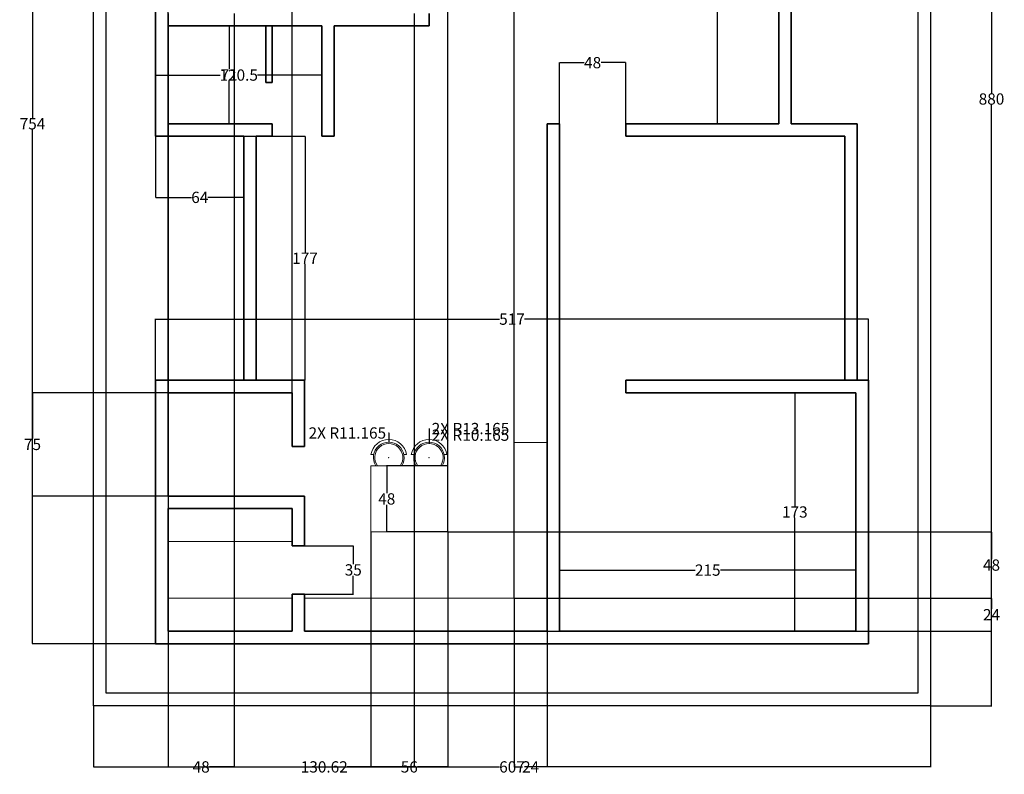
# Model space of a CAD drawing. Units: inches. Extents: x -254 to 1961, y 86 to 3025.
# Tile 5 of 6: x 1247 to 1961, y 2046 to 2593. Entities that reach past the tile are written whole.
import ezdxf

# ---------------------------------------------------------------- set-up
doc = ezdxf.new("R2010")
doc.units = ezdxf.units.IN
doc.header["$MEASUREMENT"] = 0
for name, color, linetype, lineweight in [('A-ANNO-DIMS', 2, 'Continuous', 18), ('C-SITE-WALL', 8, 'Continuous', 30), ('FURNITURE', 151, 'Continuous', 13), ('KITCHEN', 9, 'Continuous', 18), ('WALLS', 255, 'Continuous', 35)]:
    doc.layers.add(name, color=color, linetype=linetype, lineweight=lineweight)
doc.styles.get("Standard").update_dxf_attribs({"font": 'arial.ttf'})
doc.dimstyles.get("Standard").update_dxf_attribs({"dimtxt": 8.18, "dimasz": 0.18, "dimexe": 0.18, "dimexo": 0.0625, "dimgap": 0.09, "dimtad": 0, "dimtih": 1, "dimtoh": 1, "dimdec": 1, "dimzin": 0, "dimdsep": 46, "dimlunit": 3, "dimtxsty": 'Standard', "dimcen": 0.09, "dimadec": 0, "dimazin": 0, "dimtfac": 1, "dimtdec": 1, "dimtofl": 0, "dimtmove": 0, "dimatfit": 3, "dimfxl": 1, "dimtolj": 1, "dimtzin": 0, "dimarcsym": 0})

# ---------------------------------------------------------------- blocks, each defined once
blk = doc.blocks.new('*D71')
at = {"layer": 'A-ANNO-DIMS', "color": 0, "lineweight": -2, "transparency": 16777216}
for p, q in [((1300.37, 2095.39), (1300.37, 2050.93)), ((1907.37, 2095.39), (1907.37, 2050.93)), ((1300.55, 2051.11), (1594.72, 2051.11)), ((1907.19, 2051.11), (1613.02, 2051.11))]:
    blk.add_line(p, q, dxfattribs=at)
at = {"layer": 'A-ANNO-DIMS', "color": 0, "transparency": 16777216}
for points in [[(1300.55, 2051.14), (1300.55, 2051.08), (1300.37, 2051.11)], [(1907.19, 2051.14), (1907.19, 2051.08), (1907.37, 2051.11)]]:
    blk.add_solid(points, dxfattribs=at)
at = {"layer": 'Defpoints', "color": 0, "transparency": 16777216}
for p in [(1300.37, 2095.46), (1907.37, 2095.46), (1907.37, 2051.11)]:
    blk.add_point(p, dxfattribs=at)
at = {"layer": 'A-ANNO-DIMS', "color": 0, "transparency": 16777216, "insert": (1603.87, 2051.11), "char_height": 8.18, "attachment_point": 5}
blk.add_mtext('\\A1;607', dxfattribs=at)
blk = doc.blocks.new('*D72')
at = {"layer": 'A-ANNO-DIMS', "color": 0, "lineweight": -2, "transparency": 16777216}
for p, q in [((1907.43, 2975.46), (1951.9, 2975.46)), ((1951.72, 2975.28), (1951.72, 2539.72)), ((1951.72, 2095.64), (1951.72, 2531.19)), ((1907.43, 2095.46), (1951.9, 2095.46))]:
    blk.add_line(p, q, dxfattribs=at)
at = {"layer": 'A-ANNO-DIMS', "color": 0, "transparency": 16777216}
for points in [[(1951.69, 2975.28), (1951.75, 2975.28), (1951.72, 2975.46)], [(1951.69, 2095.64), (1951.75, 2095.64), (1951.72, 2095.46)]]:
    blk.add_solid(points, dxfattribs=at)
at = {"layer": 'Defpoints', "color": 0, "transparency": 16777216}
for p in [(1907.37, 2975.46), (1951.72, 2975.46), (1907.37, 2095.46)]:
    blk.add_point(p, dxfattribs=at)
at = {"layer": 'A-ANNO-DIMS', "color": 0, "transparency": 16777216, "insert": (1951.72, 2535.46), "char_height": 8.18, "attachment_point": 5}
blk.add_mtext('\\A1;880', dxfattribs=at)
blk = doc.blocks.new('*D73')
at = {"layer": 'A-ANNO-DIMS', "color": 0, "lineweight": -2, "transparency": 16777216}
for p, q in [((1345.37, 2331.52), (1345.37, 2375.99)), ((1345.55, 2375.81), (1594.74, 2375.81)), ((1862.19, 2375.81), (1613, 2375.81)), ((1862.37, 2331.52), (1862.37, 2375.99))]:
    blk.add_line(p, q, dxfattribs=at)
at = {"layer": 'A-ANNO-DIMS', "color": 0, "transparency": 16777216}
for points in [[(1345.55, 2375.84), (1345.55, 2375.78), (1345.37, 2375.81)], [(1862.19, 2375.84), (1862.19, 2375.78), (1862.37, 2375.81)]]:
    blk.add_solid(points, dxfattribs=at)
at = {"layer": 'Defpoints', "color": 0, "transparency": 16777216}
for p in [(1862.37, 2375.81), (1345.37, 2331.46), (1862.37, 2331.46)]:
    blk.add_point(p, dxfattribs=at)
at = {"layer": 'A-ANNO-DIMS', "color": 0, "transparency": 16777216, "insert": (1603.87, 2375.81), "char_height": 8.18, "attachment_point": 5}
blk.add_mtext('\\A1;517', dxfattribs=at)
blk = doc.blocks.new('*D74')
at = {"layer": 'A-ANNO-DIMS', "color": 0, "lineweight": -2, "transparency": 16777216}
for p, q in [((1345.31, 2894.46), (1255.84, 2894.46)), ((1256.02, 2894.28), (1256.02, 2521.71)), ((1256.02, 2140.64), (1256.02, 2513.21)), ((1345.31, 2140.46), (1255.84, 2140.46))]:
    blk.add_line(p, q, dxfattribs=at)
at = {"layer": 'A-ANNO-DIMS', "color": 0, "transparency": 16777216}
for points in [[(1255.99, 2894.28), (1256.05, 2894.28), (1256.02, 2894.46)], [(1255.99, 2140.64), (1256.05, 2140.64), (1256.02, 2140.46)]]:
    blk.add_solid(points, dxfattribs=at)
at = {"layer": 'Defpoints', "color": 0, "transparency": 16777216}
for p in [(1256.02, 2894.46), (1345.37, 2894.46), (1345.37, 2140.46)]:
    blk.add_point(p, dxfattribs=at)
at = {"layer": 'A-ANNO-DIMS', "color": 0, "transparency": 16777216, "insert": (1256.02, 2517.46), "char_height": 8.18, "attachment_point": 5}
blk.add_mtext('\\A1;754', dxfattribs=at)
blk = doc.blocks.new('*D87')
at = {"layer": 'A-ANNO-DIMS', "color": 0, "lineweight": -2, "transparency": 16777216}
for p, q in [((1797.31, 2753.46), (1752.84, 2753.46)), ((1753.02, 2753.28), (1753.02, 2639.72)), ((1753.02, 2517.64), (1753.02, 2631.19)), ((1797.31, 2517.46), (1752.84, 2517.46))]:
    blk.add_line(p, q, dxfattribs=at)
at = {"layer": 'A-ANNO-DIMS', "color": 0, "transparency": 16777216}
for points in [[(1752.99, 2753.28), (1753.05, 2753.28), (1753.02, 2753.46)], [(1752.99, 2517.64), (1753.05, 2517.64), (1753.02, 2517.46)]]:
    blk.add_solid(points, dxfattribs=at)
at = {"layer": 'Defpoints', "color": 0, "transparency": 16777216}
for p in [(1753.02, 2753.46), (1797.37, 2753.46), (1797.37, 2517.46)]:
    blk.add_point(p, dxfattribs=at)
at = {"layer": 'A-ANNO-DIMS', "color": 0, "transparency": 16777216, "insert": (1753.02, 2635.46), "char_height": 8.18, "attachment_point": 5}
blk.add_mtext('\\A1;236', dxfattribs=at)
blk = doc.blocks.new('*D88')
at = {"layer": 'A-ANNO-DIMS', "color": 0, "lineweight": -2, "transparency": 16777216}
for p, q in [((1409.43, 2508.46), (1453.9, 2508.46)), ((1453.72, 2508.28), (1453.72, 2424.15)), ((1453.72, 2331.64), (1453.72, 2415.76)), ((1409.43, 2331.46), (1453.9, 2331.46))]:
    blk.add_line(p, q, dxfattribs=at)
at = {"layer": 'A-ANNO-DIMS', "color": 0, "transparency": 16777216}
for points in [[(1453.69, 2508.28), (1453.75, 2508.28), (1453.72, 2508.46)], [(1453.69, 2331.64), (1453.75, 2331.64), (1453.72, 2331.46)]]:
    blk.add_solid(points, dxfattribs=at)
at = {"layer": 'Defpoints', "color": 0, "transparency": 16777216}
for p in [(1409.37, 2508.46), (1409.37, 2331.46), (1453.72, 2331.46)]:
    blk.add_point(p, dxfattribs=at)
at = {"layer": 'A-ANNO-DIMS', "color": 0, "transparency": 16777216, "insert": (1453.72, 2419.96), "char_height": 8.18, "attachment_point": 5}
blk.add_mtext('\\A1;177', dxfattribs=at)
blk = doc.blocks.new('*D89')
at = {"layer": 'A-ANNO-DIMS', "color": 0, "lineweight": -2, "transparency": 16777216}
for p, q in [((1345.37, 2508.39), (1345.37, 2463.93)), ((1409.37, 2508.39), (1409.37, 2463.93)), ((1345.55, 2464.11), (1371.41, 2464.11)), ((1409.19, 2464.11), (1383.32, 2464.11))]:
    blk.add_line(p, q, dxfattribs=at)
at = {"layer": 'A-ANNO-DIMS', "color": 0, "transparency": 16777216}
for points in [[(1345.55, 2464.14), (1345.55, 2464.08), (1345.37, 2464.11)], [(1409.19, 2464.14), (1409.19, 2464.08), (1409.37, 2464.11)]]:
    blk.add_solid(points, dxfattribs=at)
at = {"layer": 'Defpoints', "color": 0, "transparency": 16777216}
for p in [(1345.37, 2508.46), (1409.37, 2508.46), (1345.37, 2464.11)]:
    blk.add_point(p, dxfattribs=at)
at = {"layer": 'A-ANNO-DIMS', "color": 0, "transparency": 16777216, "insert": (1377.37, 2464.11), "char_height": 8.18, "attachment_point": 5}
blk.add_mtext('\\A1;64', dxfattribs=at)
blk = doc.blocks.new('*D90')
at = {"layer": 'A-ANNO-DIMS', "color": 0, "lineweight": -2, "transparency": 16777216}
for p, q in [((1638.37, 2149.52), (1638.37, 2193.99)), ((1638.55, 2193.81), (1736.64, 2193.81)), ((1853.19, 2193.81), (1755.1, 2193.81)), ((1853.37, 2149.52), (1853.37, 2193.99))]:
    blk.add_line(p, q, dxfattribs=at)
at = {"layer": 'A-ANNO-DIMS', "color": 0, "transparency": 16777216}
for points in [[(1638.55, 2193.84), (1638.55, 2193.78), (1638.37, 2193.81)], [(1853.19, 2193.84), (1853.19, 2193.78), (1853.37, 2193.81)]]:
    blk.add_solid(points, dxfattribs=at)
at = {"layer": 'Defpoints', "color": 0, "transparency": 16777216}
for p in [(1853.37, 2193.81), (1638.37, 2149.46), (1853.37, 2149.46)]:
    blk.add_point(p, dxfattribs=at)
at = {"layer": 'A-ANNO-DIMS', "color": 0, "transparency": 16777216, "insert": (1745.87, 2193.81), "char_height": 8.18, "attachment_point": 5}
blk.add_mtext('\\A1;215', dxfattribs=at)
blk = doc.blocks.new('*D91')
at = {"layer": 'A-ANNO-DIMS', "color": 0, "lineweight": -2, "transparency": 16777216}
for p, q in [((1853.31, 2322.46), (1808.84, 2322.46)), ((1809.02, 2322.28), (1809.02, 2240.22)), ((1809.02, 2149.64), (1809.02, 2231.69)), ((1853.31, 2149.46), (1808.84, 2149.46))]:
    blk.add_line(p, q, dxfattribs=at)
at = {"layer": 'A-ANNO-DIMS', "color": 0, "transparency": 16777216}
for points in [[(1808.99, 2322.28), (1809.05, 2322.28), (1809.02, 2322.46)], [(1808.99, 2149.64), (1809.05, 2149.64), (1809.02, 2149.46)]]:
    blk.add_solid(points, dxfattribs=at)
at = {"layer": 'Defpoints', "color": 0, "transparency": 16777216}
for p in [(1809.02, 2322.46), (1853.37, 2322.46), (1853.37, 2149.46)]:
    blk.add_point(p, dxfattribs=at)
at = {"layer": 'A-ANNO-DIMS', "color": 0, "transparency": 16777216, "insert": (1809.02, 2235.96), "char_height": 8.18, "attachment_point": 5}
blk.add_mtext('\\A1;173', dxfattribs=at)
blk = doc.blocks.new('*D92')
at = {"layer": 'A-ANNO-DIMS', "color": 0, "lineweight": -2, "transparency": 16777216}
for p, q in [((1638.37, 2517.52), (1638.37, 2561.99)), ((1638.55, 2561.81), (1656.25, 2561.81)), ((1686.19, 2561.81), (1668.49, 2561.81)), ((1686.37, 2517.52), (1686.37, 2561.99))]:
    blk.add_line(p, q, dxfattribs=at)
at = {"layer": 'A-ANNO-DIMS', "color": 0, "transparency": 16777216}
for points in [[(1638.55, 2561.84), (1638.55, 2561.78), (1638.37, 2561.81)], [(1686.19, 2561.84), (1686.19, 2561.78), (1686.37, 2561.81)]]:
    blk.add_solid(points, dxfattribs=at)
at = {"layer": 'Defpoints', "color": 0, "transparency": 16777216}
for p in [(1686.37, 2561.81), (1638.37, 2517.46), (1686.37, 2517.46)]:
    blk.add_point(p, dxfattribs=at)
at = {"layer": 'A-ANNO-DIMS', "color": 0, "transparency": 16777216, "insert": (1662.37, 2561.81), "char_height": 8.18, "attachment_point": 5}
blk.add_mtext('\\A1;48', dxfattribs=at)
blk = doc.blocks.new('*D93')
at = {"layer": 'A-ANNO-DIMS', "color": 0, "lineweight": -2, "transparency": 16777216}
for p, q in [((1402.37, 2597.39), (1402.37, 2050.93)), ((1532.98, 2597.39), (1532.98, 2050.93)), ((1402.55, 2051.11), (1451.03, 2051.11)), ((1532.8, 2051.11), (1484.32, 2051.11))]:
    blk.add_line(p, q, dxfattribs=at)
at = {"layer": 'A-ANNO-DIMS', "color": 0, "transparency": 16777216}
for points in [[(1402.55, 2051.14), (1402.55, 2051.08), (1402.37, 2051.11)], [(1532.8, 2051.14), (1532.8, 2051.08), (1532.98, 2051.11)]]:
    blk.add_solid(points, dxfattribs=at)
at = {"layer": 'Defpoints', "color": 0, "transparency": 16777216}
for p in [(1402.37, 2597.46), (1532.98, 2597.46), (1532.98, 2051.11)]:
    blk.add_point(p, dxfattribs=at)
at = {"layer": 'A-ANNO-DIMS', "color": 0, "transparency": 16777216, "insert": (1467.68, 2051.11), "char_height": 8.18, "attachment_point": 5}
blk.add_mtext('\\A1;130.62', dxfattribs=at)
blk = doc.blocks.new('*D94')
at = {"layer": 'A-ANNO-DIMS', "color": 0, "lineweight": -2, "transparency": 16777216}
for p, q in [((1354.37, 2597.39), (1354.37, 2050.93)), ((1402.37, 2597.39), (1402.37, 2050.93)), ((1354.55, 2051.11), (1372.25, 2051.11)), ((1402.19, 2051.11), (1384.49, 2051.11))]:
    blk.add_line(p, q, dxfattribs=at)
at = {"layer": 'A-ANNO-DIMS', "color": 0, "transparency": 16777216}
for points in [[(1354.55, 2051.14), (1354.55, 2051.08), (1354.37, 2051.11)], [(1402.19, 2051.14), (1402.19, 2051.08), (1402.37, 2051.11)]]:
    blk.add_solid(points, dxfattribs=at)
at = {"layer": 'Defpoints', "color": 0, "transparency": 16777216}
for p in [(1354.37, 2597.46), (1402.37, 2597.46), (1402.37, 2051.11)]:
    blk.add_point(p, dxfattribs=at)
at = {"layer": 'A-ANNO-DIMS', "color": 0, "transparency": 16777216, "insert": (1378.37, 2051.11), "char_height": 8.18, "attachment_point": 5}
blk.add_mtext('\\A1;48', dxfattribs=at)
blk = doc.blocks.new('*D99')
at = {"layer": 'A-ANNO-DIMS', "color": 0, "lineweight": -2, "transparency": 16777216}
for p, q in [((1345.37, 2508.52), (1345.37, 2552.99)), ((1345.55, 2552.81), (1392.08, 2552.81)), ((1465.69, 2552.81), (1419.16, 2552.81)), ((1465.87, 2508.52), (1465.87, 2552.99))]:
    blk.add_line(p, q, dxfattribs=at)
at = {"layer": 'A-ANNO-DIMS', "color": 0, "transparency": 16777216}
for points in [[(1345.55, 2552.84), (1345.55, 2552.78), (1345.37, 2552.81)], [(1465.69, 2552.84), (1465.69, 2552.78), (1465.87, 2552.81)]]:
    blk.add_solid(points, dxfattribs=at)
at = {"layer": 'Defpoints', "color": 0, "transparency": 16777216}
for p in [(1465.87, 2552.81), (1345.37, 2508.46), (1465.87, 2508.46)]:
    blk.add_point(p, dxfattribs=at)
at = {"layer": 'A-ANNO-DIMS', "color": 0, "transparency": 16777216, "insert": (1405.62, 2552.81), "char_height": 8.18, "attachment_point": 5}
blk.add_mtext('\\A1;120.5', dxfattribs=at)
blk = doc.blocks.new('*D100')
at = {"layer": 'A-ANNO-DIMS', "color": 0, "lineweight": -2, "transparency": 16777216}
for p, q in [((1354.43, 2588.46), (1398.9, 2588.46)), ((1398.72, 2588.28), (1398.72, 2557.15)), ((1398.72, 2517.64), (1398.72, 2548.76)), ((1354.43, 2517.46), (1398.9, 2517.46))]:
    blk.add_line(p, q, dxfattribs=at)
at = {"layer": 'A-ANNO-DIMS', "color": 0, "transparency": 16777216}
for points in [[(1398.69, 2588.28), (1398.75, 2588.28), (1398.72, 2588.46)], [(1398.69, 2517.64), (1398.75, 2517.64), (1398.72, 2517.46)]]:
    blk.add_solid(points, dxfattribs=at)
at = {"layer": 'Defpoints', "color": 0, "transparency": 16777216}
for p in [(1354.37, 2588.46), (1354.37, 2517.46), (1398.72, 2517.46)]:
    blk.add_point(p, dxfattribs=at)
at = {"layer": 'A-ANNO-DIMS', "color": 0, "transparency": 16777216, "insert": (1398.72, 2552.96), "char_height": 8.18, "attachment_point": 5}
blk.add_mtext('\\A1;71', dxfattribs=at)
blk = doc.blocks.new('*D104')
at = {"layer": 'A-ANNO-DIMS', "color": 0, "lineweight": -2, "transparency": 16777216}
for p, q in [((1354.37, 2322.52), (1354.37, 3019.99)), ((1354.55, 3019.81), (1393.43, 3019.81)), ((1444.19, 3019.81), (1405.3, 3019.81)), ((1444.37, 2322.52), (1444.37, 3019.99))]:
    blk.add_line(p, q, dxfattribs=at)
at = {"layer": 'A-ANNO-DIMS', "color": 0, "transparency": 16777216}
for points in [[(1354.55, 3019.84), (1354.55, 3019.78), (1354.37, 3019.81)], [(1444.19, 3019.84), (1444.19, 3019.78), (1444.37, 3019.81)]]:
    blk.add_solid(points, dxfattribs=at)
at = {"layer": 'Defpoints', "color": 0, "transparency": 16777216}
for p in [(1444.37, 3019.81), (1354.37, 2322.46), (1444.37, 2322.46)]:
    blk.add_point(p, dxfattribs=at)
at = {"layer": 'A-ANNO-DIMS', "color": 0, "transparency": 16777216, "insert": (1399.37, 3019.81), "char_height": 8.18, "attachment_point": 5}
blk.add_mtext('\\A1;90', dxfattribs=at)
blk = doc.blocks.new('*D105')
at = {"layer": 'A-ANNO-DIMS', "color": 0, "lineweight": -2, "transparency": 16777216}
for p, q in [((1354.31, 2322.46), (1255.84, 2322.46)), ((1256.02, 2322.28), (1256.02, 2289.21)), ((1256.02, 2247.64), (1256.02, 2280.71)), ((1354.31, 2247.46), (1255.84, 2247.46))]:
    blk.add_line(p, q, dxfattribs=at)
at = {"layer": 'A-ANNO-DIMS', "color": 0, "transparency": 16777216}
for points in [[(1255.99, 2322.28), (1256.05, 2322.28), (1256.02, 2322.46)], [(1255.99, 2247.64), (1256.05, 2247.64), (1256.02, 2247.46)]]:
    blk.add_solid(points, dxfattribs=at)
at = {"layer": 'Defpoints', "color": 0, "transparency": 16777216}
for p in [(1256.02, 2322.46), (1354.37, 2322.46), (1354.37, 2247.46)]:
    blk.add_point(p, dxfattribs=at)
at = {"layer": 'A-ANNO-DIMS', "color": 0, "transparency": 16777216, "insert": (1256.02, 2284.96), "char_height": 8.18, "attachment_point": 5}
blk.add_mtext('\\A1;75', dxfattribs=at)
blk = doc.blocks.new('*D106')
at = {"layer": 'A-ANNO-DIMS', "color": 0, "lineweight": -2, "transparency": 16777216}
for p, q in [((1444.43, 2211.46), (1488.9, 2211.46)), ((1488.72, 2211.28), (1488.72, 2198.22)), ((1488.72, 2176.64), (1488.72, 2189.69)), ((1444.43, 2176.46), (1488.9, 2176.46))]:
    blk.add_line(p, q, dxfattribs=at)
at = {"layer": 'A-ANNO-DIMS', "color": 0, "transparency": 16777216}
for points in [[(1488.69, 2211.28), (1488.75, 2211.28), (1488.72, 2211.46)], [(1488.69, 2176.64), (1488.75, 2176.64), (1488.72, 2176.46)]]:
    blk.add_solid(points, dxfattribs=at)
at = {"layer": 'Defpoints', "color": 0, "transparency": 16777216}
for p in [(1444.37, 2211.46), (1444.37, 2176.46), (1488.72, 2176.46)]:
    blk.add_point(p, dxfattribs=at)
at = {"layer": 'A-ANNO-DIMS', "color": 0, "transparency": 16777216, "insert": (1488.72, 2193.96), "char_height": 8.18, "attachment_point": 5}
blk.add_mtext('\\A1;35', dxfattribs=at)
blk = doc.blocks.new('*D107')
at = {"layer": 'A-ANNO-DIMS', "color": 0, "lineweight": -2, "transparency": 16777216}
for p, q in [((1605.37, 2173.39), (1605.37, 2050.93)), ((1629.37, 2149.39), (1629.37, 2050.93)), ((1605.55, 2051.11), (1611.37, 2051.11)), ((1629.19, 2051.11), (1623.37, 2051.11))]:
    blk.add_line(p, q, dxfattribs=at)
at = {"layer": 'A-ANNO-DIMS', "color": 0, "transparency": 16777216}
for points in [[(1605.55, 2051.14), (1605.55, 2051.08), (1605.37, 2051.11)], [(1629.19, 2051.14), (1629.19, 2051.08), (1629.37, 2051.11)]]:
    blk.add_solid(points, dxfattribs=at)
at = {"layer": 'Defpoints', "color": 0, "transparency": 16777216}
for p in [(1605.37, 2173.46), (1629.37, 2149.46), (1629.37, 2051.11)]:
    blk.add_point(p, dxfattribs=at)
at = {"layer": 'A-ANNO-DIMS', "color": 0, "transparency": 16777216, "insert": (1617.37, 2051.11), "char_height": 8.18, "attachment_point": 5}
blk.add_mtext('\\A1;24', dxfattribs=at)
blk = doc.blocks.new('*D108')
at = {"layer": 'A-ANNO-DIMS', "color": 0, "lineweight": -2, "transparency": 16777216}
for p, q in [((1605.43, 2173.46), (1951.9, 2173.46)), ((1951.72, 2173.28), (1951.72, 2165.65)), ((1951.72, 2149.64), (1951.72, 2157.26)), ((1629.43, 2149.46), (1951.9, 2149.46))]:
    blk.add_line(p, q, dxfattribs=at)
at = {"layer": 'A-ANNO-DIMS', "color": 0, "transparency": 16777216}
for points in [[(1951.69, 2173.28), (1951.75, 2173.28), (1951.72, 2173.46)], [(1951.69, 2149.64), (1951.75, 2149.64), (1951.72, 2149.46)]]:
    blk.add_solid(points, dxfattribs=at)
at = {"layer": 'Defpoints', "color": 0, "transparency": 16777216}
for p in [(1605.37, 2173.46), (1629.37, 2149.46), (1951.72, 2149.46)]:
    blk.add_point(p, dxfattribs=at)
at = {"layer": 'A-ANNO-DIMS', "color": 0, "transparency": 16777216, "insert": (1951.72, 2161.46), "char_height": 8.18, "attachment_point": 5}
blk.add_mtext('\\A1;24', dxfattribs=at)
blk = doc.blocks.new('*D109')
at = {"layer": 'A-ANNO-DIMS', "color": 0, "lineweight": -2, "transparency": 16777216}
for p, q in [((1501.37, 2221.39), (1501.37, 2050.93)), ((1557.37, 2221.39), (1557.37, 2050.93)), ((1501.55, 2051.11), (1523.42, 2051.11)), ((1557.19, 2051.11), (1535.32, 2051.11))]:
    blk.add_line(p, q, dxfattribs=at)
at = {"layer": 'A-ANNO-DIMS', "color": 0, "transparency": 16777216}
for points in [[(1501.55, 2051.14), (1501.55, 2051.08), (1501.37, 2051.11)], [(1557.19, 2051.14), (1557.19, 2051.08), (1557.37, 2051.11)]]:
    blk.add_solid(points, dxfattribs=at)
at = {"layer": 'Defpoints', "color": 0, "transparency": 16777216}
for p in [(1501.37, 2221.46), (1557.37, 2221.46), (1557.37, 2051.11)]:
    blk.add_point(p, dxfattribs=at)
at = {"layer": 'A-ANNO-DIMS', "color": 0, "transparency": 16777216, "insert": (1529.37, 2051.11), "char_height": 8.18, "attachment_point": 5}
blk.add_mtext('\\A1;56', dxfattribs=at)
blk = doc.blocks.new('*D110')
at = {"layer": 'A-ANNO-DIMS', "color": 0, "lineweight": -2, "transparency": 16777216}
for p, q in [((1557.31, 2269.46), (1512.84, 2269.46)), ((1513.02, 2269.28), (1513.02, 2249.72)), ((1513.02, 2221.64), (1513.02, 2241.19)), ((1557.31, 2221.46), (1512.84, 2221.46))]:
    blk.add_line(p, q, dxfattribs=at)
at = {"layer": 'A-ANNO-DIMS', "color": 0, "transparency": 16777216}
for points in [[(1512.99, 2269.28), (1513.05, 2269.28), (1513.02, 2269.46)], [(1512.99, 2221.64), (1513.05, 2221.64), (1513.02, 2221.46)]]:
    blk.add_solid(points, dxfattribs=at)
at = {"layer": 'Defpoints', "color": 0, "transparency": 16777216}
for p in [(1513.02, 2269.46), (1557.37, 2269.46), (1557.37, 2221.46)]:
    blk.add_point(p, dxfattribs=at)
at = {"layer": 'A-ANNO-DIMS', "color": 0, "transparency": 16777216, "insert": (1513.02, 2245.46), "char_height": 8.18, "attachment_point": 5}
blk.add_mtext('\\A1;48', dxfattribs=at)
blk = doc.blocks.new('*D111')
at = {"layer": 'A-ANNO-DIMS', "color": 0, "lineweight": -2, "transparency": 16777216}
for p, q in [((1557.37, 2221.52), (1557.37, 3019.99)), ((1557.55, 3019.81), (1575.25, 3019.81)), ((1605.19, 3019.81), (1587.49, 3019.81)), ((1605.37, 2173.52), (1605.37, 3019.99))]:
    blk.add_line(p, q, dxfattribs=at)
at = {"layer": 'A-ANNO-DIMS', "color": 0, "transparency": 16777216}
for points in [[(1557.55, 3019.84), (1557.55, 3019.78), (1557.37, 3019.81)], [(1605.19, 3019.84), (1605.19, 3019.78), (1605.37, 3019.81)]]:
    blk.add_solid(points, dxfattribs=at)
at = {"layer": 'Defpoints', "color": 0, "transparency": 16777216}
for p in [(1605.37, 3019.81), (1557.37, 2221.46), (1605.37, 2173.46)]:
    blk.add_point(p, dxfattribs=at)
at = {"layer": 'A-ANNO-DIMS', "color": 0, "transparency": 16777216, "insert": (1581.37, 3019.81), "char_height": 8.18, "attachment_point": 5}
blk.add_mtext('\\A1;48', dxfattribs=at)
blk = doc.blocks.new('*D112')
at = {"layer": 'A-ANNO-DIMS', "color": 0, "lineweight": -2, "transparency": 16777216}
for p, q in [((1557.43, 2221.46), (1951.9, 2221.46)), ((1951.72, 2221.28), (1951.72, 2201.72)), ((1951.72, 2173.64), (1951.72, 2193.19)), ((1605.43, 2173.46), (1951.9, 2173.46))]:
    blk.add_line(p, q, dxfattribs=at)
at = {"layer": 'A-ANNO-DIMS', "color": 0, "transparency": 16777216}
for points in [[(1951.69, 2221.28), (1951.75, 2221.28), (1951.72, 2221.46)], [(1951.69, 2173.64), (1951.75, 2173.64), (1951.72, 2173.46)]]:
    blk.add_solid(points, dxfattribs=at)
at = {"layer": 'Defpoints', "color": 0, "transparency": 16777216}
for p in [(1557.37, 2221.46), (1605.37, 2173.46), (1951.72, 2173.46)]:
    blk.add_point(p, dxfattribs=at)
at = {"layer": 'A-ANNO-DIMS', "color": 0, "transparency": 16777216, "insert": (1951.72, 2197.46), "char_height": 8.18, "attachment_point": 5}
blk.add_mtext('\\A1;48', dxfattribs=at)
blk = doc.blocks.new('*D115')
at = {"layer": 'A-ANNO-DIMS', "color": 0, "lineweight": -2, "transparency": 16777216}
for p, q in [((1543.89, 2296.46), (1543.71, 2296.46)), ((1543.71, 2296.46), (1543.71, 2288.74)), ((1543.62, 2275.39), (1543.8, 2275.39)), ((1543.71, 2275.3), (1543.71, 2275.48))]:
    blk.add_line(p, q, dxfattribs=at)
at = {"layer": 'A-ANNO-DIMS', "color": 0, "transparency": 16777216}
blk.add_solid([(1543.68, 2288.74), (1543.74, 2288.74), (1543.71, 2288.56)], dxfattribs=at)
at = {"layer": 'Defpoints', "color": 0, "transparency": 16777216}
for p in [(1543.71, 2288.56), (1543.71, 2275.39)]:
    blk.add_point(p, dxfattribs=at)
at = {"layer": 'A-ANNO-DIMS', "color": 0, "transparency": 16777216, "insert": (1573.76, 2296.46), "char_height": 8.18, "attachment_point": 5}
blk.add_mtext('\\A1;2X R13.165', dxfattribs=at)
blk = doc.blocks.new('*D116')
at = {"layer": 'A-ANNO-DIMS', "color": 0, "lineweight": -2, "transparency": 16777216}
for p, q in [((1514.3, 2293.25), (1514.48, 2293.25)), ((1514.48, 2293.25), (1514.48, 2286.74)), ((1514.39, 2275.39), (1514.57, 2275.39)), ((1514.48, 2275.3), (1514.48, 2275.48))]:
    blk.add_line(p, q, dxfattribs=at)
at = {"layer": 'A-ANNO-DIMS', "color": 0, "transparency": 16777216}
blk.add_solid([(1514.51, 2286.74), (1514.45, 2286.74), (1514.48, 2286.56)], dxfattribs=at)
at = {"layer": 'Defpoints', "color": 0, "transparency": 16777216}
for p in [(1514.48, 2286.56), (1514.48, 2275.39)]:
    blk.add_point(p, dxfattribs=at)
at = {"layer": 'A-ANNO-DIMS', "color": 0, "transparency": 16777216, "insert": (1484.42, 2293.25), "char_height": 8.18, "attachment_point": 5}
blk.add_mtext('\\A1;2X R11.165', dxfattribs=at)
blk = doc.blocks.new('*D117')
at = {"layer": 'A-ANNO-DIMS', "color": 0, "lineweight": -2, "transparency": 16777216}
for p, q in [((1543.89, 2291.66), (1543.71, 2291.66)), ((1543.71, 2291.66), (1543.71, 2285.74)), ((1543.62, 2275.39), (1543.8, 2275.39)), ((1543.71, 2275.3), (1543.71, 2275.48))]:
    blk.add_line(p, q, dxfattribs=at)
at = {"layer": 'A-ANNO-DIMS', "color": 0, "transparency": 16777216}
blk.add_solid([(1543.68, 2285.74), (1543.74, 2285.74), (1543.71, 2285.56)], dxfattribs=at)
at = {"layer": 'Defpoints', "color": 0, "transparency": 16777216}
for p in [(1543.71, 2285.56), (1543.71, 2275.39)]:
    blk.add_point(p, dxfattribs=at)
at = {"layer": 'A-ANNO-DIMS', "color": 0, "transparency": 16777216, "insert": (1573.76, 2291.66), "char_height": 8.18, "attachment_point": 5}
blk.add_mtext('\\A1;2X R10.165', dxfattribs=at)

msp = doc.modelspace()

# ---------------------------------------------------------------- linework, layer by layer
at = {"layer": 'C-SITE-WALL'}
for points in [[(1300.3694, 2975.4553), (1907.3694, 2975.4553), (1907.3694, 2095.4553), (1300.3694, 2095.4553)], [(1309.3694, 2966.4553), (1898.3694, 2966.4553), (1898.3694, 2104.4553), (1309.3694, 2104.4553)]]:
    msp.add_lwpolyline(points, close=True, dxfattribs=at)
at = {"layer": 'FURNITURE'}
for points in [[(1525.4101, 2277.6516), (1527.4459, 2277.6516, 0.8407694), (1501.507, 2277.6516), (1503.5427, 2277.6516)], [(1554.6435, 2277.6516), (1556.6792, 2277.6516, 0.8408323), (1530.74, 2277.6516), (1532.7757, 2277.6516)]]:
    msp.add_lwpolyline(points, format="xyb", dxfattribs=at)
msp.add_lwpolyline([(1501.3694, 2221.4553), (1557.3694, 2221.4553), (1557.3694, 2269.4553), (1501.3694, 2269.4553)], close=True, dxfattribs=at)
for centre, radius, start, end in [((1514.4764, 2275.3909), 11.165, 327.8847209, 212.1152791), ((1543.7096, 2275.3918), 11.165, 327.878929, 212.121071), ((1514.4764, 2275.3909), 10.165, 324.27299, 215.72701), ((1543.7096, 2275.3918), 10.165, 324.2663527, 215.7336473)]:
    msp.add_arc(centre, radius, start, end, dxfattribs=at)
at = {"layer": 'KITCHEN'}
for p, q in [((1354.3694, 2214.4553), (1444.3694, 2214.4553)), ((1354.3694, 2173.4553), (1444.3694, 2173.4553))]:
    msp.add_line(p, q, dxfattribs=at)
msp.add_lwpolyline([(1453.3694, 2173.4553), (1605.3694, 2173.4553), (1605.3694, 2286.4553), (1629.3694, 2286.4553)], dxfattribs=at)
at = {"layer": 'WALLS'}
for p, q in [((1345.3694, 2508.4553), (1345.3694, 2894.4553)), ((1797.3694, 2517.4553), (1797.3694, 2753.4553)), ((1806.3694, 2517.4553), (1806.3694, 2753.4553)), ((1543.8694, 2588.4553), (1543.8694, 2597.4553)), ((1354.3694, 2517.4553), (1354.3694, 2588.4553)), ((1354.3694, 2588.4553), (1465.8694, 2588.4553)), ((1425.3694, 2547.4553), (1425.3694, 2588.4553)), ((1429.8694, 2547.4553), (1429.8694, 2588.4553)), ((1465.8694, 2508.4553), (1465.8694, 2588.4553)), ((1474.8694, 2508.4553), (1474.8694, 2588.4553)), ((1474.8694, 2588.4553), (1543.8694, 2588.4553)), ((1425.3694, 2547.4553), (1429.8694, 2547.4553)), ((1354.3694, 2517.4553), (1429.8694, 2517.4553)), ((1429.8694, 2508.4553), (1429.8694, 2517.4553)), ((1629.3694, 2149.4553), (1629.3694, 2517.4553)), ((1629.3694, 2517.4553), (1638.3694, 2517.4553)), ((1638.3694, 2149.4553), (1638.3694, 2517.4553)), ((1686.3694, 2517.4553), (1797.3694, 2517.4553)), ((1686.3694, 2508.4553), (1686.3694, 2517.4553)), ((1806.3694, 2517.4553), (1854.3694, 2517.4553)), ((1854.3694, 2331.4553), (1854.3694, 2517.4553)), ((1345.3694, 2508.4553), (1409.3694, 2508.4553)), ((1409.3694, 2331.4553), (1409.3694, 2508.4553)), ((1418.3694, 2331.4553), (1418.3694, 2508.4553)), ((1418.3694, 2508.4553), (1429.8694, 2508.4553)), ((1465.8694, 2508.4553), (1474.8694, 2508.4553)), ((1686.3694, 2508.4553), (1845.3694, 2508.4553)), ((1845.3694, 2331.4553), (1845.3694, 2508.4553)), ((1345.3694, 2140.4553), (1345.3694, 2331.4553)), ((1345.3694, 2331.4553), (1453.3694, 2331.4553)), ((1453.3694, 2283.4553), (1453.3694, 2331.4553)), ((1686.3694, 2331.4553), (1862.3694, 2331.4553)), ((1686.3694, 2322.4553), (1686.3694, 2331.4553)), ((1862.3694, 2140.4553), (1862.3694, 2331.4553)), ((1354.3694, 2322.4553), (1444.3694, 2322.4553)), ((1354.3694, 2247.4553), (1354.3694, 2322.4553)), ((1444.3694, 2283.4553), (1444.3694, 2322.4553)), ((1686.3694, 2322.4553), (1853.3694, 2322.4553)), ((1853.3694, 2149.4553), (1853.3694, 2322.4553)), ((1444.3694, 2283.4553), (1453.3694, 2283.4553)), ((1354.3694, 2247.4553), (1453.3694, 2247.4553)), ((1453.3694, 2211.4553), (1453.3694, 2247.4553)), ((1354.3694, 2149.4553), (1354.3694, 2238.4553)), ((1354.3694, 2238.4553), (1444.3694, 2238.4553)), ((1444.3694, 2211.4553), (1444.3694, 2238.4553)), ((1444.3694, 2211.4553), (1453.3694, 2211.4553)), ((1444.3694, 2149.4553), (1444.3694, 2176.4553)), ((1444.3694, 2176.4553), (1453.3694, 2176.4553)), ((1453.3694, 2149.4553), (1453.3694, 2176.4553)), ((1354.3694, 2149.4553), (1444.3694, 2149.4553)), ((1453.3694, 2149.4553), (1629.3694, 2149.4553)), ((1638.3694, 2149.4553), (1853.3694, 2149.4553)), ((1345.3694, 2140.4553), (1862.3694, 2140.4553))]:
    msp.add_line(p, q, dxfattribs=at)

# ---------------------------------------------------------------- dimensions: what is measured, and where the dimension line sits
at = {"layer": 'A-ANNO-DIMS'}
for base, p1, p2, override, picture, middle in [((1444.3694, 3019.8053), (1354.3694, 2322.4553), (1444.3694, 2322.4553), {"dimdec": 0, "dimlfac": 1, "dimrnd": 0, "dimzin": 0, "dimdsep": 46, "dimlunit": 2}, '*D104', (1399.3694, 3019.8053)), ((1605.3694, 3019.8053), (1557.3694, 2221.4553), (1605.3694, 2173.4553), {"dimdec": 0, "dimlfac": 1, "dimrnd": 0, "dimzin": 0, "dimdsep": 46, "dimlunit": 2}, '*D111', (1581.3694, 3019.8053)), ((1402.3694, 2051.1053), (1354.3694, 2597.4553), (1402.3694, 2597.4553), {"dimdec": 0, "dimlfac": 1, "dimrnd": 0, "dimzin": 0, "dimdsep": 46, "dimlunit": 2}, '*D94', (1378.3694, 2051.1053)), ((1532.9848, 2051.1053), (1402.3694, 2597.4553), (1532.9848, 2597.4553), {"dimdec": 2, "dimlfac": 1, "dimrnd": 0, "dimzin": 0, "dimdsep": 46, "dimlunit": 2}, '*D93', (1467.6771, 2051.1053)), ((1686.3694, 2561.8053), (1638.3694, 2517.4553), (1686.3694, 2517.4553), {"dimdec": 0, "dimlfac": 1, "dimrnd": 0, "dimzin": 0, "dimdsep": 46, "dimlunit": 2}, '*D92', (1662.3694, 2561.8053)), ((1862.3694, 2375.8053), (1345.3694, 2331.4553), (1862.3694, 2331.4553), {"dimdec": 0, "dimlfac": 1, "dimrnd": 0, "dimzin": 0, "dimdsep": 46, "dimlunit": 2}, '*D73', (1603.8694, 2375.8053)), ((1557.3694, 2051.1053), (1501.3694, 2221.4553), (1557.3694, 2221.4553), {"dimdec": 0, "dimlfac": 1, "dimrnd": 0, "dimzin": 0, "dimdsep": 46, "dimlunit": 2}, '*D109', (1529.3694, 2051.1053)), ((1853.3694, 2193.8053), (1638.3694, 2149.4553), (1853.3694, 2149.4553), {"dimdec": 0, "dimlfac": 1, "dimrnd": 0, "dimzin": 0, "dimdsep": 46, "dimlunit": 2}, '*D90', (1745.8694, 2193.8053)), ((1629.3694, 2051.1053), (1605.3694, 2173.4553), (1629.3694, 2149.4553), {"dimdec": 0, "dimlfac": 1, "dimrnd": 0, "dimzin": 0, "dimdsep": 46, "dimlunit": 2}, '*D107', (1617.3694, 2051.1053)), ((1907.3694, 2051.1053), (1300.3694, 2095.4553), (1907.3694, 2095.4553), {"dimdec": 0, "dimlfac": 1, "dimrnd": 0, "dimzin": 0, "dimdsep": 46, "dimlunit": 2}, '*D71', (1603.8694, 2051.1053))]:
    dim = msp.add_linear_dim(base=base, p1=p1, p2=p2, dimstyle='Standard', override=override, dxfattribs=at)
    dim.commit()
    dim.dimension.update_dxf_attribs({"geometry": picture, "text_midpoint": middle})
for base, p1, p2, angle, override, picture, middle in [((1951.7194, 2975.4553), (1907.3694, 2095.4553), (1907.3694, 2975.4553), 90, {"dimdec": 0, "dimlfac": 1, "dimrnd": 0, "dimzin": 0, "dimdsep": 46, "dimlunit": 2}, '*D72', (1951.7194, 2535.4553)), ((1256.0194, 2894.4553), (1345.3694, 2140.4553), (1345.3694, 2894.4553), 90, {"dimdec": 0, "dimlfac": 1, "dimrnd": 0, "dimzin": 0, "dimdsep": 46, "dimlunit": 2}, '*D74', (1256.0194, 2517.4553)), ((1753.0194, 2753.4553), (1797.3694, 2517.4553), (1797.3694, 2753.4553), 90, {"dimdec": 0, "dimlfac": 1, "dimrnd": 0, "dimzin": 0, "dimdsep": 46, "dimlunit": 2}, '*D87', (1753.0194, 2635.4553)), ((1398.7194, 2517.4553), (1354.3694, 2588.4553), (1354.3694, 2517.4553), 270, {"dimdec": 0, "dimlfac": 1, "dimrnd": 0, "dimzin": 0, "dimdsep": 46, "dimlunit": 2}, '*D100', (1398.7194, 2552.9553)), ((1465.8694, 2552.8053), (1345.3694, 2508.4553), (1465.8694, 2508.4553), 0, {"dimdec": 1, "dimlfac": 1, "dimrnd": 0, "dimzin": 0, "dimdsep": 46, "dimlunit": 2}, '*D99', (1405.6194, 2552.8053)), ((1345.3694, 2464.1053), (1409.3694, 2508.4553), (1345.3694, 2508.4553), 180, {"dimdec": 0, "dimlfac": 1, "dimrnd": 0, "dimzin": 0, "dimdsep": 46, "dimlunit": 2}, '*D89', (1377.3694, 2464.1053)), ((1453.7194, 2331.4553), (1409.3694, 2508.4553), (1409.3694, 2331.4553), 270, {"dimdec": 0, "dimlfac": 1, "dimrnd": 0, "dimzin": 0, "dimdsep": 46, "dimlunit": 2}, '*D88', (1453.7194, 2419.9553)), ((1256.0194, 2322.4553), (1354.3694, 2247.4553), (1354.3694, 2322.4553), 90, {"dimdec": 0, "dimlfac": 1, "dimrnd": 0, "dimzin": 0, "dimdsep": 46, "dimlunit": 2}, '*D105', (1256.0194, 2284.9553)), ((1809.0194, 2322.4553), (1853.3694, 2149.4553), (1853.3694, 2322.4553), 90, {"dimdec": 0, "dimlfac": 1, "dimrnd": 0, "dimzin": 0, "dimdsep": 46, "dimlunit": 2}, '*D91', (1809.0194, 2235.9553)), ((1513.0194, 2269.4553), (1557.3694, 2221.4553), (1557.3694, 2269.4553), 90, {"dimdec": 0, "dimlfac": 1, "dimrnd": 0, "dimzin": 0, "dimdsep": 46, "dimlunit": 2}, '*D110', (1513.0194, 2245.4553)), ((1951.7194, 2173.4553), (1557.3694, 2221.4553), (1605.3694, 2173.4553), 90, {"dimdec": 0, "dimlfac": 1, "dimrnd": 0, "dimzin": 0, "dimdsep": 46, "dimlunit": 2}, '*D112', (1951.7194, 2197.4553)), ((1488.7194, 2176.4553), (1444.3694, 2211.4553), (1444.3694, 2176.4553), 270, {"dimdec": 0, "dimlfac": 1, "dimrnd": 0, "dimzin": 0, "dimdsep": 46, "dimlunit": 2}, '*D106', (1488.7194, 2193.9553)), ((1951.7194, 2149.4553), (1605.3694, 2173.4553), (1629.3694, 2149.4553), 90, {"dimdec": 0, "dimlfac": 1, "dimrnd": 0, "dimzin": 0, "dimdsep": 46, "dimlunit": 2}, '*D108', (1951.7194, 2161.4553))]:
    dim = msp.add_linear_dim(base=base, p1=p1, p2=p2, angle=angle, dimstyle='Standard', override=override, dxfattribs=at)
    dim.commit()
    dim.dimension.update_dxf_attribs({"geometry": picture, "text_midpoint": middle})
for center, mpoint, picture, middle in [((1543.7096, 2275.3918), (1543.71, 2288.5568), '*D115', (1573.7625, 2296.4558)), ((1514.4764, 2275.3909), (1514.476, 2286.5559), '*D116', (1484.4235, 2293.2549)), ((1543.7096, 2275.3918), (1543.71, 2285.5568), '*D117', (1573.7625, 2291.6558))]:
    dim = msp.add_radius_dim(center=center, mpoint=mpoint, text='2X <>', dimstyle='Standard', override={"dimdec": 3, "dimlfac": 1, "dimrnd": 0, "dimzin": 0, "dimdsep": 46, "dimlunit": 2}, dxfattribs=at)
    dim.commit()
    dim.dimension.update_dxf_attribs({"geometry": picture, "text_midpoint": middle, "dimtype": 164})

doc.saveas('drawing.dxf')
